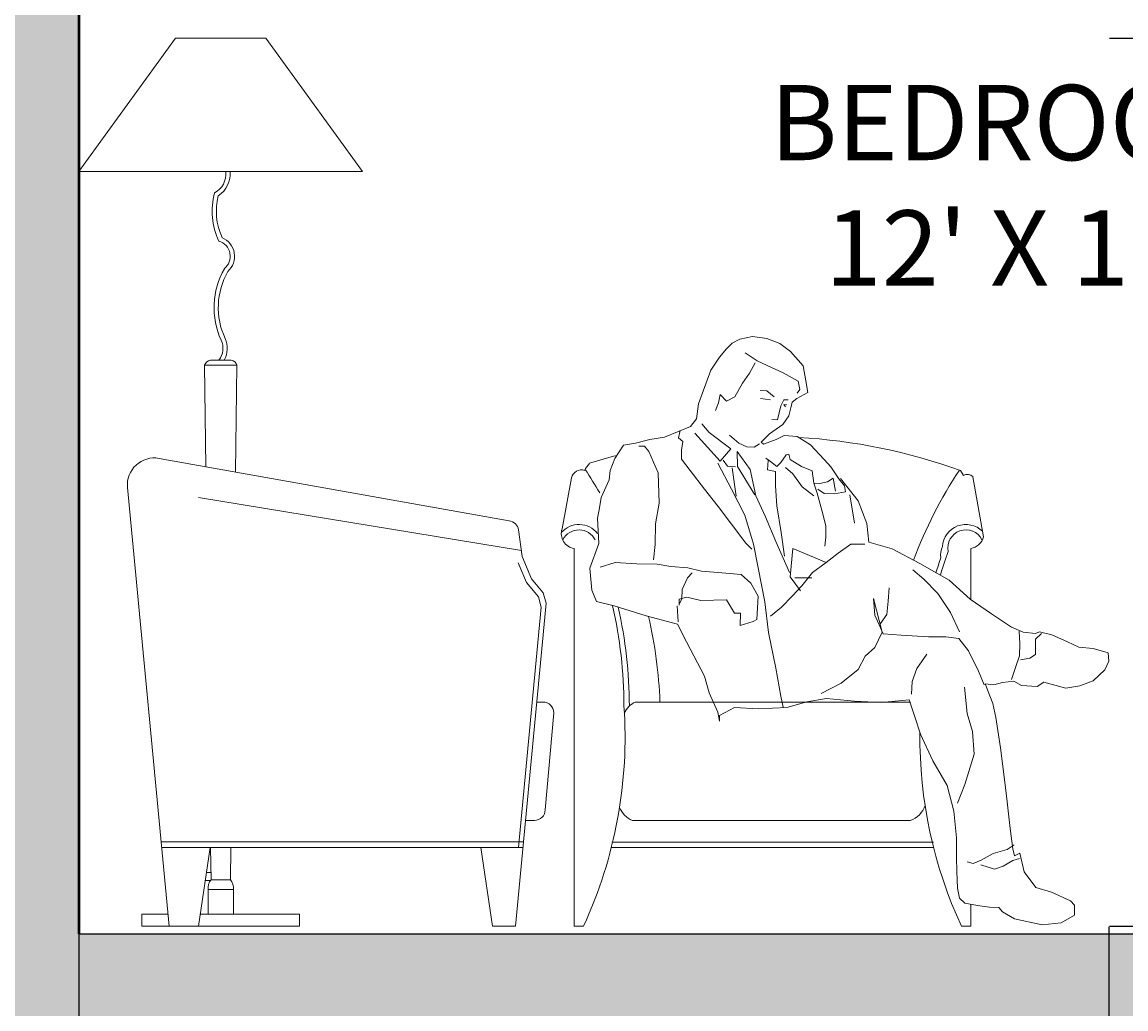
# Model space of a CAD drawing. Units: inches. Extents: x 1771 to 3025, y 319 to 889.
# Tile 15 of 35: x 2402 to 2505, y 473 to 564. Entities that reach past the tile are written whole.
import ezdxf

# ---------------------------------------------------------------- set-up
doc = ezdxf.new("R2010")
doc.units = ezdxf.units.IN
doc.header["$MEASUREMENT"] = 0
for name, color, linetype, lineweight in [('A-ANNO-DIMS', 2, 'Continuous', 18), ('A-AREA-IDEN', 241, 'Continuous', 25), ('A-FLOR-STRS', 7, 'Continuous', 25), ('A-FURN', 8, 'Continuous', 18), ('A-WALL', 7, 'Continuous', 50), ('A-WALL-PATT', 254, 'Continuous', 13)]:
    doc.layers.add(name, color=color, linetype=linetype, lineweight=lineweight)
doc.styles.get("Standard").update_dxf_attribs({"font": 'arial.ttf'})
doc.dimstyles.get("Standard").update_dxf_attribs({"dimtxt": 0.18, "dimasz": 0.18, "dimexe": 0.18, "dimexo": 0.0625, "dimgap": 0.09, "dimtad": 0, "dimtih": 1, "dimtoh": 1, "dimdec": 4, "dimzin": 0, "dimdsep": 46, "dimtxsty": 'Standard', "dimcen": 0.09, "dimadec": 0, "dimazin": 0, "dimtfac": 1, "dimtdec": 4, "dimtofl": 0, "dimtmove": 0, "dimatfit": 3, "dimfxl": 1, "dimtolj": 1, "dimtzin": 0, "dimarcsym": 0})

# ---------------------------------------------------------------- blocks, each defined once
blk = doc.blocks.new('A$C0DCF6C46')
for p, q in [((179.4, 1650), (0, 1402.3)), ((179.4, 1650), (0, 1402.3)), ((179.4, 1650), (347.3, 1650)), ((179.4, 1650), (347.3, 1650)), ((347.3, 1650), (526.7, 1402.3)), ((347.3, 1650), (526.7, 1402.3)), ((0, 1402.3), (526.7, 1402.3)), ((0, 1402.3), (526.7, 1402.3)), ((1213.4, 1083.3), (1227.6, 1090.4)), ((1213.4, 1083.3), (1227.6, 1090.4)), ((1227.6, 1090.4), (1251, 1095.4)), ((1227.6, 1090.4), (1251, 1095.4)), ((1251, 1095.4), (1277.5, 1092)), ((1251, 1095.4), (1277.5, 1092)), ((1277.5, 1092), (1301.8, 1082.8)), ((1277.5, 1092), (1301.8, 1082.8)), ((1189.7, 1057.2), (1202.6, 1072.4)), ((1189.7, 1057.2), (1202.6, 1072.4)), ((1202.6, 1072.4), (1213.4, 1083.3)), ((1202.6, 1072.4), (1213.4, 1083.3)), ((1301.8, 1082.8), (1321.9, 1067.8)), ((1301.8, 1082.8), (1321.9, 1067.8)), ((1321.9, 1067.8), (1345.5, 1041.1)), ((1321.9, 1067.8), (1345.5, 1041.1)), ((244, 1051.7), (282.6, 1051.7)), ((244, 1051.7), (282.6, 1051.7)), ((1173.6, 1032.9), (1189.7, 1057.2)), ((1173.6, 1032.9), (1189.7, 1057.2)), ((1259.7, 1050.3), (1237.5, 1065.3)), ((1259.7, 1050.3), (1237.5, 1065.3)), ((1255.9, 1046.6), (1245.7, 1027.6)), ((1255.9, 1046.6), (1245.7, 1027.6)), ((1278.7, 1041.6), (1259.7, 1050.3)), ((1278.7, 1041.6), (1259.7, 1050.3)), ((233.4, 1042.3), (293.3, 1042.3)), ((233.4, 1042.3), (235.7, 853.7)), ((233.4, 1042.3), (293.3, 1042.3)), ((233.4, 1042.3), (235.7, 853.7)), ((293.3, 1042.3), (290.8, 843.9)), ((293.3, 1042.3), (290.8, 843.9)), ((1150.8, 970.5), (1173.6, 1032.9)), ((1150.8, 970.5), (1173.6, 1032.9)), ((1245.7, 1027.6), (1232.3, 1009.1)), ((1245.7, 1027.6), (1232.3, 1009.1)), ((1308.3, 1028.1), (1278.7, 1041.6)), ((1308.3, 1028.1), (1278.7, 1041.6)), ((1335.8, 1012.5), (1308.3, 1028.1)), ((1335.8, 1012.5), (1308.3, 1028.1)), ((1345.5, 1041.1), (1350.1, 1013.5)), ((1345.5, 1041.1), (1350.1, 1013.5)), ((1232.3, 1009.1), (1218.3, 983.7)), ((1232.3, 1009.1), (1218.3, 983.7)), ((1338.8, 997.1), (1335.8, 1012.5)), ((1338.8, 997.1), (1335.8, 1012.5)), ((1350.1, 1013.5), (1354.2, 991.7)), ((1350.1, 1013.5), (1354.2, 991.7)), ((1190.8, 987.7), (1188, 972.3)), ((1190.8, 987.7), (1188, 972.3)), ((1202.9, 975.4), (1190.8, 987.7)), ((1202.9, 975.4), (1190.8, 987.7)), ((1277.8, 994.4), (1265.6, 995)), ((1277.8, 994.4), (1265.6, 995)), ((1291.5, 983.2), (1277.8, 994.4)), ((1291.5, 983.2), (1277.8, 994.4)), ((1354.2, 991.7), (1333.4, 980.2)), ((1354.2, 991.7), (1333.4, 980.2)), ((1334, 990.3), (1338.8, 997.1)), ((1334, 990.3), (1338.8, 997.1)), ((1147.4, 942.9), (1150.8, 970.5)), ((1147.4, 942.9), (1150.8, 970.5)), ((1188, 972.3), (1182.6, 958)), ((1188, 972.3), (1182.6, 958)), ((1218.3, 983.7), (1202.9, 975.4)), ((1218.3, 983.7), (1202.9, 975.4)), ((1266, 980.7), (1284.6, 977.9)), ((1266, 980.7), (1284.6, 977.9)), ((1304.1, 966.6), (1297.6, 940.6)), ((1304.1, 966.6), (1297.6, 940.6)), ((1309.5, 977.7), (1304.1, 966.6)), ((1309.5, 977.7), (1304.1, 966.6)), ((1309.4, 969), (1312.6, 964.7)), ((1314.7, 968.9), (1309.4, 969)), ((1309.4, 969), (1312.6, 964.7)), ((1314.7, 968.9), (1309.4, 969)), ((1317.5, 977.7), (1309.5, 977.7)), ((1317.5, 977.7), (1309.5, 977.7)), ((1324.9, 973.9), (1322.1, 963.3)), ((1324.9, 973.9), (1322.1, 963.3)), ((1333.4, 980.2), (1324.9, 973.9)), ((1333.4, 980.2), (1324.9, 973.9)), ((1318.8, 948.5), (1307.6, 932.1)), ((1318.8, 948.5), (1307.6, 932.1)), ((1322.1, 963.3), (1318.8, 948.5)), ((1322.1, 963.3), (1318.8, 948.5)), ((1087.8, 908.4), (1135.7, 928.2)), ((1087.8, 908.4), (1135.7, 928.2)), ((1135.7, 928.2), (1147.4, 942.9)), ((1135.7, 928.2), (1147.4, 942.9)), ((1170.4, 917.1), (1156.8, 933.1)), ((1170.4, 917.1), (1156.8, 933.1)), ((1307.6, 932.1), (1282.5, 914.8)), ((1307.6, 932.1), (1282.5, 914.8)), ((1297.6, 940.6), (1286.8, 941.4)), ((1297.6, 940.6), (1286.8, 941.4)), ((1033.6, 897.7), (1060.7, 904.4)), ((1033.6, 897.7), (1060.7, 904.4)), ((1060.7, 904.4), (1087.8, 908.4)), ((1060.7, 904.4), (1087.8, 908.4)), ((1117, 920.9), (1113.7, 907.1)), ((1117, 920.9), (1113.7, 907.1)), ((1113.7, 907.1), (1121.7, 900.7)), ((1113.7, 907.1), (1121.7, 900.7)), ((1190.9, 864.1), (1144, 915.9)), ((1190.9, 864.1), (1144, 915.9)), ((1211.2, 886.7), (1170.4, 917.1)), ((1211.2, 886.7), (1170.4, 917.1)), ((1225.9, 897.6), (1208.3, 912.3)), ((1225.9, 897.6), (1208.3, 912.3)), ((1282.5, 914.8), (1267, 899.5)), ((1282.5, 914.8), (1267, 899.5)), ((1271.7, 895.8), (1295.1, 904.1)), ((1271.7, 895.8), (1295.1, 904.1)), ((1295.1, 904.1), (1310, 911.9)), ((1295.1, 904.1), (1310, 911.9)), ((1310, 911.9), (1334.4, 909.6)), ((1310, 911.9), (1334.4, 909.6)), ((1334.4, 909.6), (1359.2, 894.6)), ((1334.4, 909.6), (1359.2, 894.6)), ((995.7, 868.8), (1011.8, 893.6)), ((995.7, 868.8), (1011.8, 893.6)), ((1011.8, 893.6), (1033.6, 897.7)), ((1011.8, 893.6), (1033.6, 897.7)), ((1039.9, 891.8), (1050.5, 891.7)), ((1039.9, 891.8), (1050.5, 891.7)), ((1050.5, 891.7), (1058.4, 882.1)), ((1050.5, 891.7), (1058.4, 882.1)), ((1058.4, 882.1), (1076.1, 842.2)), ((1058.4, 882.1), (1076.1, 842.2)), ((1119.4, 884.3), (1119.3, 867.8)), ((1119.4, 884.3), (1119.3, 867.8)), ((1121.7, 900.7), (1119.4, 884.3)), ((1121.7, 900.7), (1119.4, 884.3)), ((1211.2, 886.7), (1190.9, 864.1)), ((1211.2, 886.7), (1190.9, 864.1)), ((1222.8, 881.9), (1223.6, 853.9)), ((1247, 848.8), (1222.8, 881.9)), ((1222.8, 881.9), (1223.6, 853.9)), ((1247, 848.8), (1222.8, 881.9)), ((1240.6, 890.8), (1225.9, 897.6)), ((1240.6, 890.8), (1225.9, 897.6)), ((1254.3, 890.2), (1240.6, 890.8)), ((1254.3, 890.2), (1240.6, 890.8)), ((1264.4, 895.9), (1254.3, 890.2)), ((1264.4, 895.9), (1254.3, 890.2)), ((1267, 899.5), (1271.7, 895.8)), ((1267, 899.5), (1271.7, 895.8)), ((1359.2, 894.6), (1384, 866.8)), ((1359.2, 894.6), (1384, 866.8)), ((148.7, 869.2), (799.3, 753.3)), ((148.7, 869.2), (799.3, 753.3)), ((986.5, 846.6), (995.7, 868.8)), ((986.5, 846.6), (995.7, 868.8)), ((1119.3, 867.8), (1135.5, 846.5)), ((1119.3, 867.8), (1135.5, 846.5)), ((1196.7, 865.6), (1204.6, 855)), ((1196.7, 865.6), (1204.6, 855)), ((1275.8, 869.8), (1284.7, 863.3)), ((1275.8, 869.8), (1284.7, 863.3)), ((1278.8, 848), (1280, 865.5)), ((1278.8, 848), (1280, 865.5)), ((1284.7, 863.3), (1296.3, 854.2)), ((1284.7, 863.3), (1296.3, 854.2)), ((1296.3, 854.2), (1303.8, 861.6)), ((1296.3, 854.2), (1303.8, 861.6)), ((1303.8, 861.6), (1313.5, 875.8)), ((1303.8, 861.6), (1313.5, 875.8)), ((1313.5, 875.8), (1318.8, 876.9)), ((1313.5, 875.8), (1318.8, 876.9)), ((1318.8, 876.9), (1321.4, 867.3)), ((1318.8, 876.9), (1321.4, 867.3)), ((1321.4, 867.3), (1342.5, 854.4)), ((1321.4, 867.3), (1342.5, 854.4)), ((1384, 866.8), (1396.6, 853.4)), ((1384, 866.8), (1396.6, 853.4)), ((984.8, 829.6), (986.5, 846.6)), ((984.8, 829.6), (986.5, 846.6)), ((1076.1, 842.2), (1077.8, 785.9)), ((1076.1, 842.2), (1077.8, 785.9)), ((1135.5, 846.5), (1162.3, 812.3)), ((1135.5, 846.5), (1162.3, 812.3)), ((1186.6, 860.4), (1212.2, 811.9)), ((1186.6, 860.4), (1212.2, 811.9)), ((1204.6, 855), (1219.4, 853.2)), ((1204.6, 855), (1219.4, 853.2)), ((1213.6, 851.7), (1221.1, 799.1)), ((1213.6, 851.7), (1221.1, 799.1)), ((1223.6, 853.9), (1255.4, 801.3)), ((1223.6, 853.9), (1255.4, 801.3)), ((1257.2, 799.9), (1247, 848.8)), ((1257.2, 799.9), (1247, 848.8)), ((1293.6, 844.7), (1278.8, 848)), ((1293.6, 844.7), (1278.8, 848)), ((1293.9, 818.2), (1293.6, 844.7)), ((1293.9, 818.2), (1293.6, 844.7)), ((1325.9, 840.7), (1312.2, 852)), ((1325.9, 840.7), (1312.2, 852)), ((1342.5, 854.4), (1362, 845.8)), ((1342.5, 854.4), (1362, 845.8)), ((1362, 845.8), (1365, 822.9)), ((1362, 845.8), (1365, 822.9)), ((1396.6, 853.4), (1411.8, 831)), ((1396.6, 853.4), (1411.8, 831)), ((1637.6, 846.8), (1643.1, 837.5)), ((1637.6, 846.8), (1643.1, 837.5)), ((915.2, 833), (897.4, 738.2)), ((915.2, 833), (897.4, 738.2)), ((970.2, 796.3), (984.8, 829.6)), ((970.2, 796.3), (984.8, 829.6)), ((1343.2, 816.2), (1325.9, 840.7)), ((1343.2, 816.2), (1325.9, 840.7)), ((1376.2, 822.8), (1365, 822.9)), ((1365, 822.9), (1371.3, 804.3)), ((1376.2, 822.8), (1365, 822.9)), ((1365, 822.9), (1371.3, 804.3)), ((1390.5, 825.9), (1376.2, 822.8)), ((1390.5, 825.9), (1376.2, 822.8)), ((1401.2, 832.2), (1390.5, 825.9)), ((1401.2, 832.2), (1390.5, 825.9)), ((1405.2, 808.3), (1401.2, 832.2)), ((1405.2, 808.3), (1401.2, 832.2)), ((1411.8, 831), (1422.3, 818.2)), ((1411.8, 831), (1422.3, 818.2)), ((1414.4, 832.1), (1447.5, 790.5)), ((1414.4, 832.1), (1447.5, 790.5)), ((1680.1, 723.7), (1660.3, 834.6)), ((1680.1, 723.7), (1660.3, 834.6)), ((167.7, 0), (90.2, 815.3)), ((167.7, 0), (90.2, 815.3)), ((1162.3, 812.3), (1187.5, 779.8)), ((1162.3, 812.3), (1187.5, 779.8)), ((1212.2, 811.9), (1236.7, 763.5)), ((1212.2, 811.9), (1236.7, 763.5)), ((1275.4, 760.5), (1257.2, 799.9)), ((1275.4, 760.5), (1257.2, 799.9)), ((1296.3, 781), (1293.9, 818.2)), ((1296.3, 781), (1293.9, 818.2)), ((1364.9, 799.6), (1343.2, 816.2)), ((1364.9, 799.6), (1343.2, 816.2)), ((1371.3, 804.3), (1380.5, 770.8)), ((1371.3, 804.3), (1380.5, 770.8)), ((1384, 803.7), (1372.4, 811.7)), ((1384, 803.7), (1372.4, 811.7)), ((1403.6, 803.5), (1384, 803.7)), ((1403.6, 803.5), (1384, 803.7)), ((1423.8, 807.1), (1403.6, 803.5)), ((1423.8, 807.1), (1403.6, 803.5)), ((1422.3, 818.2), (1423.8, 807.1)), ((1422.3, 818.2), (1423.8, 807.1)), ((1431.7, 801.7), (1440.8, 748.6)), ((1431.7, 801.7), (1440.8, 748.6)), ((821.8, 697.8), (222.3, 796.3)), ((821.8, 697.8), (222.3, 796.3)), ((966.3, 773.5), (970.2, 796.3)), ((966.3, 773.5), (970.2, 796.3)), ((1077.8, 785.9), (1071.1, 747.3)), ((1077.8, 785.9), (1071.1, 747.3)), ((1187.5, 779.8), (1212.2, 747.2)), ((1187.5, 779.8), (1212.2, 747.2)), ((1304.4, 731.6), (1296.3, 781)), ((1304.4, 731.6), (1296.3, 781)), ((1447.5, 790.5), (1463.6, 748.4)), ((1447.5, 790.5), (1463.6, 748.4)), ((963, 758.2), (966.3, 773.5)), ((963, 758.2), (966.3, 773.5)), ((1236.7, 763.5), (1253.3, 709.8)), ((1236.7, 763.5), (1253.3, 709.8)), ((1294.7, 714.7), (1275.4, 760.5)), ((1294.7, 714.7), (1275.4, 760.5)), ((1380.5, 770.8), (1387.2, 743.7)), ((1380.5, 770.8), (1387.2, 743.7)), ((965.8, 711), (963, 758.2)), ((965.8, 711), (963, 758.2)), ((1071.1, 747.3), (1070.3, 709.1)), ((1071.1, 747.3), (1070.3, 709.1)), ((1212.2, 747.2), (1239, 712)), ((1212.2, 747.2), (1239, 712)), ((1387.2, 743.7), (1387.1, 723)), ((1387.2, 743.7), (1387.1, 723)), ((1463.6, 748.4), (1467.1, 713.4)), ((1463.6, 748.4), (1467.1, 713.4)), ((816.5, 736.2), (823.2, 687.2)), ((816.5, 736.2), (823.2, 687.2)), ((1310.9, 687.6), (1304.4, 731.6)), ((1310.9, 687.6), (1304.4, 731.6)), ((1387.1, 723), (1385.3, 706.1)), ((1387.1, 723), (1385.3, 706.1)), ((919.8, 701.9), (919.8, 0)), ((919.8, 701.9), (919.8, 0)), ((949, 665.5), (965.8, 711)), ((949, 665.5), (965.8, 711)), ((1070.3, 709.1), (1067.4, 681)), ((1070.3, 709.1), (1067.4, 681)), ((1239, 712), (1250, 700.8)), ((1239, 712), (1250, 700.8)), ((1253.3, 709.8), (1262, 665.7)), ((1253.3, 709.8), (1262, 665.7)), ((1319.7, 657.3), (1294.7, 714.7)), ((1319.7, 657.3), (1294.7, 714.7)), ((1325.9, 701.8), (1321.2, 649.3)), ((1325.9, 701.8), (1321.2, 649.3)), ((1387.8, 675.8), (1325.9, 701.8)), ((1387.8, 675.8), (1325.9, 701.8)), ((1410.2, 693.1), (1433.6, 709.9)), ((1410.2, 693.1), (1433.6, 709.9)), ((1433.6, 709.9), (1459.6, 709.7)), ((1433.6, 709.9), (1459.6, 709.7)), ((1467.1, 713.4), (1510.5, 701.4)), ((1467.1, 713.4), (1510.5, 701.4)), ((1510.5, 701.4), (1562.3, 673.9)), ((1510.5, 701.4), (1562.3, 673.9)), ((1656.8, 701.9), (1656.8, 607.1)), ((1656.8, 701.9), (1656.8, 607.1)), ((823.2, 687.2), (840.7, 645.7)), ((823.2, 687.2), (840.7, 645.7)), ((1387.8, 675.8), (1410.2, 693.1)), ((1387.8, 675.8), (1410.2, 693.1)), ((816.1, 675.1), (831.6, 638.4)), ((816.1, 675.1), (831.6, 638.4)), ((952.4, 624.6), (949, 665.5)), ((952.4, 624.6), (949, 665.5)), ((968.1, 667.4), (995.8, 675.7)), ((968.1, 667.4), (995.8, 675.7)), ((995.8, 675.7), (1036.1, 673.3)), ((995.8, 675.7), (1036.1, 673.3)), ((1036.1, 673.3), (1074.2, 672.4)), ((1036.1, 673.3), (1074.2, 672.4)), ((1074.2, 672.4), (1099.7, 668.5)), ((1074.2, 672.4), (1099.7, 668.5)), ((1099.7, 668.5), (1130.9, 665.6)), ((1099.7, 668.5), (1130.9, 665.6)), ((1130.3, 647.1), (1138.8, 656.6)), ((1130.3, 647.1), (1138.8, 656.6)), ((1130.9, 665.6), (1156.4, 659.6)), ((1130.9, 665.6), (1156.4, 659.6)), ((1156.4, 659.6), (1194, 656.7)), ((1156.4, 659.6), (1194, 656.7)), ((1194, 656.7), (1230, 653.7)), ((1194, 656.7), (1230, 653.7)), ((1262, 665.7), (1274.2, 603)), ((1262, 665.7), (1274.2, 603)), ((1342.9, 632.7), (1362.7, 657.4)), ((1342.9, 632.7), (1362.7, 657.4)), ((1362.7, 657.4), (1387.8, 675.8)), ((1362.7, 657.4), (1387.8, 675.8)), ((1569.5, 644.7), (1548.9, 662.4)), ((1569.5, 644.7), (1548.9, 662.4)), ((1562.3, 673.9), (1616.6, 642.7)), ((1562.3, 673.9), (1616.6, 642.7)), ((831.6, 638.4), (853.4, 612.1)), ((831.6, 638.4), (853.4, 612.1)), ((840.7, 645.7), (862.6, 619.4)), ((840.7, 645.7), (862.6, 619.4)), ((1120.6, 625.4), (1130.3, 647.1)), ((1120.6, 625.4), (1130.3, 647.1)), ((1230, 653.7), (1248, 637.7)), ((1230, 653.7), (1248, 637.7)), ((1248, 637.7), (1261.6, 613.2)), ((1248, 637.7), (1261.6, 613.2)), ((1321.2, 649.3), (1340.1, 623.1)), ((1321.2, 649.3), (1340.1, 623.1)), ((1361.5, 647.4), (1329.7, 647.6)), ((1361.5, 647.4), (1329.7, 647.6)), ((1595.2, 618), (1569.5, 644.7)), ((1595.2, 618), (1569.5, 644.7)), ((1616.6, 642.7), (1655.6, 607.9)), ((1616.6, 642.7), (1655.6, 607.9)), ((862.6, 619.4), (867.8, 600.3)), ((862.6, 619.4), (867.8, 600.3)), ((961.2, 603.3), (952.4, 624.6)), ((961.2, 603.3), (952.4, 624.6)), ((1119.9, 607.9), (1120.6, 625.4)), ((1119.9, 607.9), (1120.6, 625.4)), ((1325.7, 613.7), (1342.9, 632.7)), ((1325.7, 613.7), (1342.9, 632.7)), ((1503.4, 603.8), (1505.1, 628.7)), ((1503.4, 603.8), (1505.1, 628.7)), ((1618.8, 582.8), (1595.2, 618)), ((1618.8, 582.8), (1595.2, 618)), ((867.8, 600.3), (810.7, 0)), ((867.8, 600.3), (810.7, 0)), ((853.4, 612.1), (858.7, 592.9)), ((853.4, 612.1), (858.7, 592.9)), ((994.1, 595.1), (961.2, 603.3)), ((994.1, 595.1), (961.2, 603.3)), ((1053.9, 576.6), (994.1, 595.1)), ((1053.9, 576.6), (994.1, 595.1)), ((1111.3, 595.2), (1113.2, 565.5)), ((1111.3, 595.2), (1113.2, 565.5)), ((1115.1, 607.9), (1115, 596.8)), ((1115.1, 607.9), (1115, 596.8)), ((1128.9, 611.5), (1115.1, 607.9)), ((1128.9, 611.5), (1115.1, 607.9)), ((1115.6, 599.4), (1119.9, 607.9)), ((1115.6, 599.4), (1119.9, 607.9)), ((1154.9, 605), (1128.9, 611.5)), ((1154.9, 605), (1128.9, 611.5)), ((1202.6, 606.7), (1154.9, 605)), ((1202.6, 606.7), (1154.9, 605)), ((1217.8, 581.7), (1202.6, 606.7)), ((1217.8, 581.7), (1202.6, 606.7)), ((1261.6, 613.2), (1259.1, 569.7)), ((1261.6, 613.2), (1259.1, 569.7)), ((1274.2, 603), (1280.6, 545.6)), ((1274.2, 603), (1280.6, 545.6)), ((1304.9, 592.7), (1325.7, 613.7)), ((1304.9, 592.7), (1325.7, 613.7)), ((1475.8, 608.8), (1478.2, 578)), ((1491.8, 546.1), (1475.8, 608.8)), ((1475.8, 608.8), (1478.2, 578)), ((1491.8, 546.1), (1475.8, 608.8)), ((1501, 578.9), (1503.4, 603.8)), ((1501, 578.9), (1503.4, 603.8)), ((1655.6, 607.9), (1695.2, 580.6)), ((1655.6, 607.9), (1695.2, 580.6)), ((858.7, 592.9), (816.6, 146.6)), ((858.7, 592.9), (816.6, 146.6)), ((1112.1, 561.3), (1053.9, 576.6)), ((1112.1, 561.3), (1053.9, 576.6)), ((1228.9, 581.6), (1217.8, 581.7)), ((1228.9, 581.6), (1217.8, 581.7)), ((1228.2, 558.8), (1228.9, 581.6)), ((1228.2, 558.8), (1228.9, 581.6)), ((1284.6, 575.8), (1304.9, 592.7)), ((1284.6, 575.8), (1304.9, 592.7)), ((1478.2, 578), (1493.9, 543.4)), ((1478.2, 578), (1493.9, 543.4)), ((1489.2, 562.6), (1501, 578.9)), ((1489.2, 562.6), (1501, 578.9)), ((1635.5, 547.1), (1618.8, 582.8)), ((1635.5, 547.1), (1618.8, 582.8)), ((1695.2, 580.6), (1732.1, 555.4)), ((1695.2, 580.6), (1732.1, 555.4)), ((1128.3, 528.3), (1112.1, 561.3)), ((1128.3, 528.3), (1112.1, 561.3)), ((1252.7, 566), (1228.2, 558.8)), ((1252.7, 566), (1228.2, 558.8)), ((1259.1, 569.7), (1252.7, 566)), ((1259.1, 569.7), (1252.7, 566)), ((1732.1, 555.4), (1753.8, 546.2)), ((1732.1, 555.4), (1753.8, 546.2)), ((1280.6, 545.6), (1294.5, 479.8)), ((1280.6, 545.6), (1294.5, 479.8)), ((1478.3, 517.6), (1491.8, 546.1)), ((1478.3, 517.6), (1491.8, 546.1)), ((1493.9, 543.4), (1527.3, 540.5)), ((1493.9, 543.4), (1527.3, 540.5)), ((1527.3, 540.5), (1578.2, 538)), ((1527.3, 540.5), (1578.2, 538)), ((1578.2, 538), (1610.5, 537.7)), ((1578.2, 538), (1610.5, 537.7)), ((1610.5, 537.7), (1634.4, 534.9)), ((1610.5, 537.7), (1634.4, 534.9)), ((1634.4, 534.9), (1652.2, 511.4)), ((1634.4, 534.9), (1652.2, 511.4)), ((1747.8, 525.5), (1746.4, 548.4)), ((1747.8, 525.5), (1746.4, 548.4)), ((1753.8, 546.2), (1776.6, 543.9)), ((1753.8, 546.2), (1776.6, 543.9)), ((1776.6, 543.9), (1784.6, 547)), ((1776.6, 543.9), (1784.6, 547)), ((1788.3, 543.8), (1777, 533.3)), ((1788.3, 543.8), (1777, 533.3)), ((1777, 533.3), (1777, 522.1)), ((1777, 533.3), (1777, 522.1)), ((1784.6, 547), (1807.3, 541.5)), ((1784.6, 547), (1807.3, 541.5)), ((1807.3, 541.5), (1836.4, 528.5)), ((1807.3, 541.5), (1836.4, 528.5)), ((1142.4, 502.7), (1128.3, 528.3)), ((1142.4, 502.7), (1128.3, 528.3)), ((1460.7, 501.8), (1478.3, 517.6)), ((1460.7, 501.8), (1478.3, 517.6)), ((1747.1, 502.7), (1747.8, 525.5)), ((1747.1, 502.7), (1747.8, 525.5)), ((1777, 522.1), (1776.8, 504.6)), ((1777, 522.1), (1776.8, 504.6)), ((1836.4, 528.5), (1857.6, 518.8)), ((1836.4, 528.5), (1857.6, 518.8)), ((1857.6, 518.8), (1884.1, 516)), ((1857.6, 518.8), (1884.1, 516)), ((1884.1, 516), (1912.1, 507.8)), ((1884.1, 516), (1912.1, 507.8)), ((1162.3, 464.9), (1142.4, 502.7)), ((1162.3, 464.9), (1142.4, 502.7)), ((1447.7, 477), (1460.7, 501.8)), ((1447.7, 477), (1460.7, 501.8)), ((1556.5, 478.8), (1575.3, 505.7)), ((1556.5, 478.8), (1575.3, 505.7)), ((1652.2, 511.4), (1671, 474.2)), ((1652.2, 511.4), (1671, 474.2)), ((1740, 481), (1747.1, 502.7)), ((1740, 481), (1747.1, 502.7)), ((1766.2, 498.3), (1749.2, 494.8)), ((1766.2, 498.3), (1749.2, 494.8)), ((1776.8, 504.6), (1766.2, 498.3)), ((1776.8, 504.6), (1766.2, 498.3)), ((1913, 492.4), (1906, 476.6)), ((1913, 492.4), (1906, 476.6)), ((1912.1, 507.8), (1913, 492.4)), ((1912.1, 507.8), (1913, 492.4)), ((1294.5, 479.8), (1303.6, 427.7)), ((1294.5, 479.8), (1303.6, 427.7)), ((1415.7, 451.8), (1447.7, 477)), ((1415.7, 451.8), (1447.7, 477)), ((1547.8, 455), (1556.5, 478.8)), ((1547.8, 455), (1556.5, 478.8)), ((1671, 474.2), (1681.4, 448.6)), ((1671, 474.2), (1681.4, 448.6)), ((1732.4, 458.3), (1740, 481)), ((1732.4, 458.3), (1740, 481)), ((1906, 476.6), (1884.1, 456)), ((1906, 476.6), (1884.1, 456)), ((1170.5, 433.5), (1162.3, 464.9)), ((1170.5, 433.5), (1162.3, 464.9)), ((1379, 432.4), (1415.7, 451.8)), ((1379, 432.4), (1415.7, 451.8)), ((1546.6, 431.1), (1547.8, 455)), ((1546.6, 431.1), (1547.8, 455)), ((1715.9, 452.6), (1699.5, 448.5)), ((1715.9, 452.6), (1699.5, 448.5)), ((1736.6, 455.1), (1715.9, 452.6)), ((1736.6, 455.1), (1715.9, 452.6)), ((1750.9, 447.5), (1736.6, 455.1)), ((1750.9, 447.5), (1736.6, 455.1)), ((1792.3, 453.6), (1780.1, 445.7)), ((1792.3, 453.6), (1780.1, 445.7)), ((1833.1, 442.1), (1792.3, 453.6)), ((1833.1, 442.1), (1792.3, 453.6)), ((1884.1, 456), (1859.1, 446.7)), ((1884.1, 456), (1859.1, 446.7)), ((1186.7, 397.9), (1170.5, 433.5)), ((1186.7, 397.9), (1170.5, 433.5)), ((1645.3, 444.1), (1649.7, 395.3)), ((1645.3, 444.1), (1649.7, 395.3)), ((1683.6, 450.7), (1697.6, 414)), ((1699.5, 448.5), (1683.6, 450.7)), ((1683.6, 450.7), (1697.6, 414)), ((1699.5, 448.5), (1683.6, 450.7)), ((1780.1, 445.7), (1750.9, 447.5)), ((1780.1, 445.7), (1750.9, 447.5)), ((1859.1, 446.7), (1833.1, 442.1)), ((1859.1, 446.7), (1833.1, 442.1)), ((862, 416.6), (851.4, 416.6)), ((862, 416.6), (851.4, 416.6)), ((1033.5, 416.6), (1544.9, 416.6)), ((1033.5, 416.6), (1544.9, 416.6)), ((1303.6, 427.7), (1308.2, 407)), ((1303.6, 427.7), (1308.2, 407)), ((1351.8, 416.7), (1315.1, 406.4)), ((1351.8, 416.7), (1315.1, 406.4)), ((1388.4, 423.3), (1351.8, 416.7)), ((1388.4, 423.3), (1351.8, 416.7)), ((1440.4, 418.1), (1388.4, 423.3)), ((1440.4, 418.1), (1388.4, 423.3)), ((1490.2, 415.6), (1440.4, 418.1)), ((1490.2, 415.6), (1440.4, 418.1)), ((1542.2, 420.5), (1490.2, 415.6)), ((1542.2, 420.5), (1490.2, 415.6)), ((1552.6, 389.1), (1542.2, 420.5)), ((1552.6, 389.1), (1542.2, 420.5)), ((1697.6, 414), (1703.2, 388)), ((1697.6, 414), (1703.2, 388)), ((882, 396.6), (866.1, 216.6)), ((882, 396.6), (866.1, 216.6)), ((1189.7, 380.9), (1186.7, 397.9)), ((1189.7, 380.9), (1186.7, 397.9)), ((1189.8, 391.5), (1189.7, 380.9)), ((1189.8, 391.5), (1189.7, 380.9)), ((1217.5, 406.6), (1189.8, 391.5)), ((1217.5, 406.6), (1189.8, 391.5)), ((1262, 404.2), (1217.5, 406.6)), ((1262, 404.2), (1217.5, 406.6)), ((1315.1, 406.4), (1262, 404.2)), ((1315.1, 406.4), (1262, 404.2)), ((1649.7, 395.3), (1660.1, 361.8)), ((1649.7, 395.3), (1660.1, 361.8)), ((1563, 357.2), (1552.6, 389.1)), ((1563, 357.2), (1552.6, 389.1)), ((1703.2, 388), (1711.8, 331.7)), ((1703.2, 388), (1711.8, 331.7)), ((1585.9, 307.2), (1563, 357.2)), ((1585.9, 307.2), (1563, 357.2)), ((1660.1, 361.8), (1662.9, 319.9)), ((1660.1, 361.8), (1662.9, 319.9)), ((1711.8, 331.7), (1721.8, 252.6)), ((1711.8, 331.7), (1721.8, 252.6)), ((1662.9, 319.9), (1645.5, 263.2)), ((1662.9, 319.9), (1645.5, 263.2)), ((1612.6, 261.4), (1585.9, 307.2)), ((1612.6, 261.4), (1585.9, 307.2)), ((1625.5, 214.1), (1612.6, 261.4)), ((1625.5, 214.1), (1612.6, 261.4)), ((1645.5, 263.2), (1632, 228.9)), ((1645.5, 263.2), (1632, 228.9)), ((1721.8, 252.6), (1729.7, 181.9)), ((1721.8, 252.6), (1729.7, 181.9)), ((1629.9, 164.2), (1625.5, 214.1)), ((1629.9, 164.2), (1625.5, 214.1)), ((846.1, 196.6), (829.9, 196.6)), ((846.1, 196.6), (829.9, 196.6)), ((1028.1, 196.6), (1544.2, 196.6)), ((1028.1, 196.6), (1544.2, 196.6)), ((1630.1, 127.6), (1629.9, 164.2)), ((1630.1, 127.6), (1629.9, 164.2)), ((1729.7, 181.9), (1734.7, 143.7)), ((1729.7, 181.9), (1734.7, 143.7)), ((825, 157.1), (152.8, 157.1)), ((825, 157.1), (152.8, 157.1)), ((825, 146.6), (153.8, 146.6)), ((825, 146.6), (153.8, 146.6)), ((243.8, 146.6), (221.9, 0)), ((243.8, 146.6), (221.9, 0)), ((244.6, 146.6), (245.3, 86.3)), ((244.6, 146.6), (245.3, 86.3)), ((282.1, 146.6), (281.3, 86.3)), ((282.1, 146.6), (281.3, 86.3)), ((746.4, 146.6), (768.4, 0)), ((746.4, 146.6), (768.4, 0)), ((989.7, 156.6), (1587.6, 156.6)), ((989.7, 156.6), (1587.6, 156.6)), ((989.7, 146.6), (1587.6, 146.6)), ((989.7, 146.6), (1587.6, 146.6)), ((1737.4, 151.1), (1724.1, 142.7)), ((1737.4, 151.1), (1724.1, 142.7)), ((1734.7, 143.7), (1737.8, 131)), ((1734.7, 143.7), (1737.8, 131)), ((1631, 102.1), (1630.1, 127.6)), ((1631, 102.1), (1630.1, 127.6)), ((1698.1, 135), (1675.7, 123)), ((1698.1, 135), (1675.7, 123)), ((1724.1, 142.7), (1698.1, 135)), ((1724.1, 142.7), (1698.1, 135)), ((1747.3, 126.1), (1735.1, 122.5)), ((1747.3, 126.1), (1735.1, 122.5)), ((1737.8, 131), (1747.9, 135.7)), ((1737.8, 131), (1747.9, 135.7)), ((1747.9, 135.7), (1755.6, 101.1)), ((1747.9, 135.7), (1755.6, 101.1)), ((1661.3, 116.7), (1650.2, 119.5)), ((1661.3, 116.7), (1650.2, 119.5)), ((1675.7, 123), (1661.3, 116.7)), ((1675.7, 123), (1661.3, 116.7)), ((1701, 106.3), (1675.6, 113.9)), ((1701, 106.3), (1675.6, 113.9)), ((1717, 111.5), (1701, 106.3)), ((1717, 111.5), (1701, 106.3)), ((1735.1, 122.5), (1717, 111.5)), ((1735.1, 122.5), (1717, 111.5)), ((234.6, 85), (244.2, 85)), ((234.6, 85), (244.2, 85)), ((236.8, 100), (245.2, 100)), ((236.8, 100), (245.2, 100)), ((245.3, 86.3), (281.3, 86.3)), ((245.3, 86.3), (281.3, 86.3)), ((1632.3, 70.8), (1631, 102.1)), ((1632.3, 70.8), (1631, 102.1)), ((1755.6, 101.1), (1777.7, 72.3)), ((1755.6, 101.1), (1777.7, 72.3)), ((239.8, 68.3), (239.8, 22.5)), ((239.8, 68.3), (286.9, 68.3)), ((239.8, 68.3), (239.8, 22.5)), ((239.8, 68.3), (286.9, 68.3)), ((286.9, 68.3), (286.9, 22.5)), ((286.9, 68.3), (286.9, 22.5)), ((1635.9, 52.2), (1632.3, 70.8)), ((1635.9, 52.2), (1632.3, 70.8)), ((1777.7, 72.3), (1806.8, 63.6)), ((1777.7, 72.3), (1806.8, 63.6)), ((1806.8, 63.6), (1841.7, 47.4)), ((1806.8, 63.6), (1841.7, 47.4)), ((1645.4, 43.1), (1635.9, 52.2)), ((1645.4, 43.1), (1635.9, 52.2)), ((1669.2, 38.7), (1645.4, 43.1)), ((1669.2, 38.7), (1645.4, 43.1)), ((1841.7, 47.4), (1849.6, 39.4)), ((1841.7, 47.4), (1849.6, 39.4)), ((116.8, 22.5), (116.8, 0)), ((116.8, 22.5), (165.6, 22.5)), ((116.8, 22.5), (116.8, 0)), ((116.8, 22.5), (165.6, 22.5)), ((225.2, 22.5), (409.9, 22.5)), ((225.2, 22.5), (409.9, 22.5)), ((409.9, 22.5), (409.9, 0)), ((409.9, 22.5), (409.9, 0)), ((1656.8, 41), (1656.8, 0)), ((1656.8, 41), (1656.8, 0)), ((1691.4, 35.3), (1669.2, 38.7)), ((1691.4, 35.3), (1669.2, 38.7)), ((1709, 35.2), (1691.4, 35.3)), ((1709, 35.2), (1691.4, 35.3)), ((1715.3, 26.6), (1709, 35.2)), ((1715.3, 26.6), (1709, 35.2)), ((1738, 13.7), (1715.3, 26.6)), ((1738, 13.7), (1715.3, 26.6)), ((1849.4, 20.8), (1824.4, 6.7)), ((1849.4, 20.8), (1824.4, 6.7)), ((1849.6, 39.4), (1849.4, 20.8)), ((1849.6, 39.4), (1849.4, 20.8)), ((1789.3, 2.7), (1738, 13.7)), ((1789.3, 2.7), (1738, 13.7)), ((1824.4, 6.7), (1789.3, 2.7)), ((1824.4, 6.7), (1789.3, 2.7)), ((116.8, 0), (409.9, 0)), ((116.8, 0), (409.9, 0)), ((919.8, 0), (937.1, 0)), ((919.8, 0), (937.1, 0)), ((1639.4, 0), (1656.8, 0)), ((1639.4, 0), (1656.8, 0))]:
    blk.add_line(p, q)
for centre, radius, start, end in [((232.2, 1398.2), 40.9, 298.591, 4.7801), ((232.2, 1398.2), 40.9, 298.591, 4.7801), ((232.2, 1398.2), 48.9, 302.7794, 4.7801), ((232.2, 1398.2), 48.9, 302.7794, 4.7801), ((374.6, 1328.2), 127.4, 164.5089, 205.7991), ((374.6, 1328.2), 127.4, 164.5089, 205.7991), ((374.6, 1328.2), 119.4, 166.0279, 204.234), ((374.6, 1328.2), 119.4, 166.0279, 204.234), ((251.6, 1244.5), 29.4, 308.7103, 73.8033), ((251.6, 1244.5), 29.4, 308.7103, 73.8033), ((251.6, 1244.5), 37.4, 311.1929, 67.9822), ((251.6, 1244.5), 37.4, 311.1929, 67.9822), ((395.6, 1149.4), 144.8, 150.115, 204.7751), ((395.6, 1149.4), 144.8, 150.115, 204.7751), ((395.6, 1149.4), 136.8, 150.7005, 204.7627), ((395.6, 1149.4), 136.8, 150.7005, 204.7627), ((231.9, 1073.6), 35.6, 321.9956, 25.2261), ((231.9, 1073.6), 35.6, 321.9956, 25.2261), ((231.9, 1073.6), 43.6, 329.6961, 25.182), ((231.9, 1073.6), 43.6, 329.6961, 25.182), ((246.1, 1038.6), 13.2, 98.8052, 163.9237), ((246.1, 1038.6), 13.2, 98.8052, 163.9237), ((280.6, 1038.6), 13.2, 16.0763, 81.1948), ((280.6, 1038.6), 13.2, 16.0763, 81.1948), ((1273.4, -169.1), 1079.2, 70.279, 86.636), ((1273.4, -169.1), 1079.2, 70.279, 86.636), ((139.9, 820), 50, 79.8912, 185.4337), ((139.9, 820), 50, 79.8912, 185.4337), ((1273.4, -169.1), 1079.2, 104.7019, 107.5271), ((1273.4, -169.1), 1079.2, 104.7019, 107.5271), ((933.1, 829.6), 18.2, 70.9411, 169.1012), ((933.1, 829.6), 18.2, 70.9411, 169.1012), ((1047.8, 778.9), 128.2, 140.7938, 148.0496), ((1047.8, 778.9), 128.2, 140.7938, 148.0496), ((241, 385.5), 838.8, 30.0042, 33.5227), ((241, 385.5), 838.8, 30.0042, 33.5227), ((2335, 385.5), 838.2, 146.5555, 159.4144), ((2335, 385.5), 838.2, 146.5555, 159.4144), ((1650.3, 825), 14.4, 42.1894, 120.2274), ((1650.3, 825), 14.4, 42.1894, 120.2274), ((796.6, 733.4), 20, 7.8584, 82.4843), ((796.6, 733.4), 20, 7.8584, 82.4843), ((929, 702.9), 43.5, 37.8135, 139.3209), ((929, 702.9), 43.5, 37.8135, 139.3209), ((1647.6, 702.9), 43.5, 45.0789, 176.3198), ((1647.6, 702.9), 43.5, 45.0789, 176.3198), ((923.6, 729.2), 27.6, 161.105, 262.178), ((923.6, 729.2), 27.6, 161.105, 262.178), ((929, 702.9), 33.5, 26.3854, 153.1276), ((929, 702.9), 33.5, 26.3854, 153.1276), ((1647.6, 702.9), 33.5, 26.8724, 191.3689), ((1647.6, 702.9), 33.5, 26.8724, 191.3689), ((1653, 729.2), 27.6, 277.822, 348.4179), ((1653, 729.2), 27.6, 277.822, 348.4179), ((1639.4, 689.8), 38.7, 155.7528, 188.1441), ((1639.4, 689.8), 38.7, 155.7528, 188.1441), ((2392.2, 407.9), 838, 160.7403, 162.7196), ((2392.2, 407.9), 838, 160.7403, 162.7196), ((2420.3, 406.7), 856.1, 160.2245, 163.3332), ((2420.3, 406.7), 856.1, 160.2245, 163.3332), ((156.3, 406.7), 856.1, 0.182, 12.766), ((156.3, 406.7), 856.1, 0.182, 12.766), ((176.7, 406.6), 845.7, 0.1617, 12.7147), ((176.7, 406.6), 845.7, 0.1617, 12.7147), ((241, 385.5), 838.8, 2.1238, 13.0913), ((241, 385.5), 838.8, 2.1238, 13.0913), ((862, 396.6), 20, 0, 90), ((862, 396.6), 20, 0, 90), ((1052.6, 376.5), 44.4, 115.3918, 154.207), ((1052.6, 376.5), 44.4, 115.3918, 154.207), ((178.3, 351), 836.1, 335.1756, 4.0003), ((178.3, 351), 836.1, 335.1756, 4.0003), ((2398.3, 351), 836.1, 179.4209, 204.8244), ((2398.3, 351), 836.1, 179.4209, 204.8244), ((846.1, 216.6), 20, 270, 0), ((846.1, 216.6), 20, 270, 0), ((1045.3, 237.5), 44.4, 202.0254, 247.0946), ((1045.3, 237.5), 44.4, 202.0254, 247.0946), ((1529.6, 238.5), 44.4, 289.1171, 341.8054), ((1529.6, 238.5), 44.4, 289.1171, 341.8054), ((262.7, 71.1), 23.1, 138.7741, 186.8798), ((262.7, 71.1), 23.1, 138.7741, 186.8798), ((263.9, 71.1), 23.1, 353.1202, 41.2259), ((263.9, 71.1), 23.1, 353.1202, 41.2259)]:
    blk.add_arc(centre, radius, start, end)
blk = doc.blocks.new('A$C4223307F')
blk.add_line((768.4, 0), (810.7, 0))
blk.add_blockref('A$C0DCF6C46', (0, 0))
blk = doc.blocks.new('A$C061F63B6')
blk.add_blockref('A$C4223307F', (0, 0))
blk = doc.blocks.new('*D42')
at = {"layer": 'A-ANNO-DIMS', "color": 0, "lineweight": -2, "transparency": 16777216}
for p, q in [((2407.16, 480.28), (2407.16, 465.79)), ((2503, 480.28), (2503, 465.79)), ((2407.34, 465.97), (2453.48, 465.97)), ((2502.82, 465.97), (2456.68, 465.97))]:
    blk.add_line(p, q, dxfattribs=at)
at = {"layer": 'A-ANNO-DIMS', "color": 0, "transparency": 16777216}
for points in [[(2407.34, 466), (2407.34, 465.94), (2407.16, 465.97)], [(2502.82, 466), (2502.82, 465.94), (2503, 465.97)]]:
    blk.add_solid(points, dxfattribs=at)
at = {"layer": 'Defpoints', "color": 0, "transparency": 16777216}
for p in [(2407.16, 480.34), (2503, 480.34), (2503, 465.97)]:
    blk.add_point(p, dxfattribs=at)
at = {"layer": 'A-ANNO-DIMS', "color": 0, "transparency": 16777216, "insert": (2455.08, 465.97), "char_height": 0.18, "attachment_point": 5}
blk.add_mtext('\\A1;LOUNGE CHAIRS 96 TYP.', dxfattribs=at)
blk = doc.blocks.new('*D43')
at = {"layer": 'A-ANNO-DIMS', "color": 0, "lineweight": -2, "transparency": 16777216}
for p, q in [((2503.06, 563), (2517.55, 563)), ((2517.37, 562.82), (2517.37, 521.86)), ((2517.37, 480.52), (2517.37, 521.49)), ((2503.06, 480.34), (2517.55, 480.34))]:
    blk.add_line(p, q, dxfattribs=at)
at = {"layer": 'A-ANNO-DIMS', "color": 0, "transparency": 16777216}
for points in [[(2517.34, 562.82), (2517.4, 562.82), (2517.37, 563)], [(2517.34, 480.52), (2517.4, 480.52), (2517.37, 480.34)]]:
    blk.add_solid(points, dxfattribs=at)
at = {"layer": 'Defpoints', "color": 0, "transparency": 16777216}
for p in [(2503, 563), (2517.37, 563), (2503, 480.34)]:
    blk.add_point(p, dxfattribs=at)
at = {"layer": 'A-ANNO-DIMS', "color": 0, "transparency": 16777216, "insert": (2517.37, 521.67), "char_height": 0.18, "attachment_point": 5}
blk.add_mtext('\\A1;83 TYP.', dxfattribs=at)

msp = doc.modelspace()

# ---------------------------------------------------------------- hatches: boundary and pattern name
at = {"layer": 'A-WALL-PATT'}
h = msp.add_hatch(color=256, dxfattribs=at)
h.dxf.hatch_style = 1
h.paths.add_polyline_path([(2407.16, 878.63), (2429.21, 878.63), (2429.21, 888.63), (2379.16, 888.63), (2379.16, 878.63), (2402.16, 878.63), (2402.16, 830.63), (2407.16, 830.63)])
h.paths.add_polyline_path([(2520.11, 888.63), (2477.21, 888.63), (2477.21, 878.63), (2498.16, 878.63), (2498.16, 794.63), (2402.16, 794.63), (2402.16, 758.63), (2402.16, 664.63), (2407.16, 664.63), (2407.16, 712), (2407.16, 789.63), (2515.16, 789.63), (2515.16, 794.63), (2503.16, 794.63), (2503.16, 878.63), (2520.11, 878.63)])
h.paths.add_polyline_path([(2561.16, 888.63), (2538.11, 888.63), (2538.11, 878.63), (2551.16, 878.63), (2551.16, 789.63), (2551.16, 768.61), (2561.16, 768.61)])
h.paths.add_polyline_path([(2561.16, 720.61), (2551.16, 720.61), (2551.16, 669.63), (2443.16, 669.63), (2443.16, 664.63), (2462.16, 664.63), (2462.16, 652.63), (2467.16, 652.63), (2467.16, 664.63), (2551.16, 664.63), (2551.16, 649.17), (2561.16, 649.17)])
h.paths.add_polyline_path([(2561.16, 631.17), (2551.16, 631.17), (2551.16, 616.63), (2462.16, 616.63), (2443.16, 616.63), (2443.16, 611.63), (2551.16, 611.63), (2551.16, 581.11), (2561.16, 581.11)])
h.paths.add_polyline_path([(2561.16, 533.11), (2551.16, 533.11), (2551.16, 479.63), (2407.16, 479.63), (2407.16, 616.63), (2397.16, 616.63), (2397.16, 543.63), (2306.16, 543.63), (2306.16, 533.63), (2397.16, 533.63), (2397.16, 469.63), (2551.16, 469.63), (2551.16, 452.76), (2561.16, 452.76)])
h.paths.add_polyline_path([(2561.16, 404.76), (2551.16, 404.76), (2551.16, 393.63), (2397.16, 393.63), (2397.16, 383.63), (2561.16, 383.63)])
h.paths.add_polyline_path([(2270.16, 642.58), (2260.16, 642.58), (2260.16, 533.63), (2270.16, 533.63)])
h.paths.add_polyline_path([(2270.16, 753.63), (2366.16, 753.63), (2366.16, 758.63), (2270.16, 758.63), (2270.16, 842.59, -0.008336), (2268.86, 842.63), (2260.16, 842.63), (2260.16, 690.58), (2270.16, 690.58)])
h.paths.add_polyline_path([(2331.16, 888.63), (2260.16, 888.63), (2260.16, 878.63), (2331.16, 878.63)])

# ---------------------------------------------------------------- linework, layer by layer
at = {"layer": 'A-FLOR-STRS'}
msp.add_line((2407.16, 479.63), (2551.16, 479.63), dxfattribs=at)
at = {"layer": 'A-WALL'}
msp.add_line((2407.16, 616.63), (2407.16, 479.63), dxfattribs=at)

# ---------------------------------------------------------------- block references
at = {"layer": 'A-FURN', "xscale": 0.0500958271542837, "yscale": 0.0500958271542837, "zscale": 0.0500958271542837}
msp.add_blockref('A$C061F63B6', (2407.16, 480.34), dxfattribs=at)

# ---------------------------------------------------------------- texts
at = {"layer": 'A-AREA-IDEN', "insert": (2451.97, 558.63), "char_height": 7, "attachment_point": 1}
msp.add_mtext_dynamic_manual_height_columns("\\pxqc;BEDROOM\\P12' X 11'", width=85.4611, gutter_width=1, heights=[0], dxfattribs=at)

# ---------------------------------------------------------------- dimensions: what is measured, and where the dimension line sits
at = {"layer": 'A-ANNO-DIMS'}
dim = msp.add_linear_dim(base=(2517.37, 563), p1=(2503, 480.34), p2=(2503, 563), angle=90, text='<> TYP.', dimstyle='Standard', override={"dimdec": 0, "dimrnd": 0, "dimzin": 0, "dimlunit": 2}, dxfattribs=at)
dim.commit()
dim.dimension.update_dxf_attribs({"geometry": '*D43', "text_midpoint": (2517.37, 521.67)})
dim = msp.add_linear_dim(base=(2503, 465.97), p1=(2407.16, 480.34), p2=(2503, 480.34), text='LOUNGE CHAIRS <> TYP.', dimstyle='Standard', override={"dimdec": 0, "dimrnd": 0, "dimzin": 0, "dimlunit": 2}, dxfattribs=at)
dim.commit()
dim.dimension.update_dxf_attribs({"geometry": '*D42', "text_midpoint": (2455.08, 465.97)})

doc.saveas('drawing.dxf')
